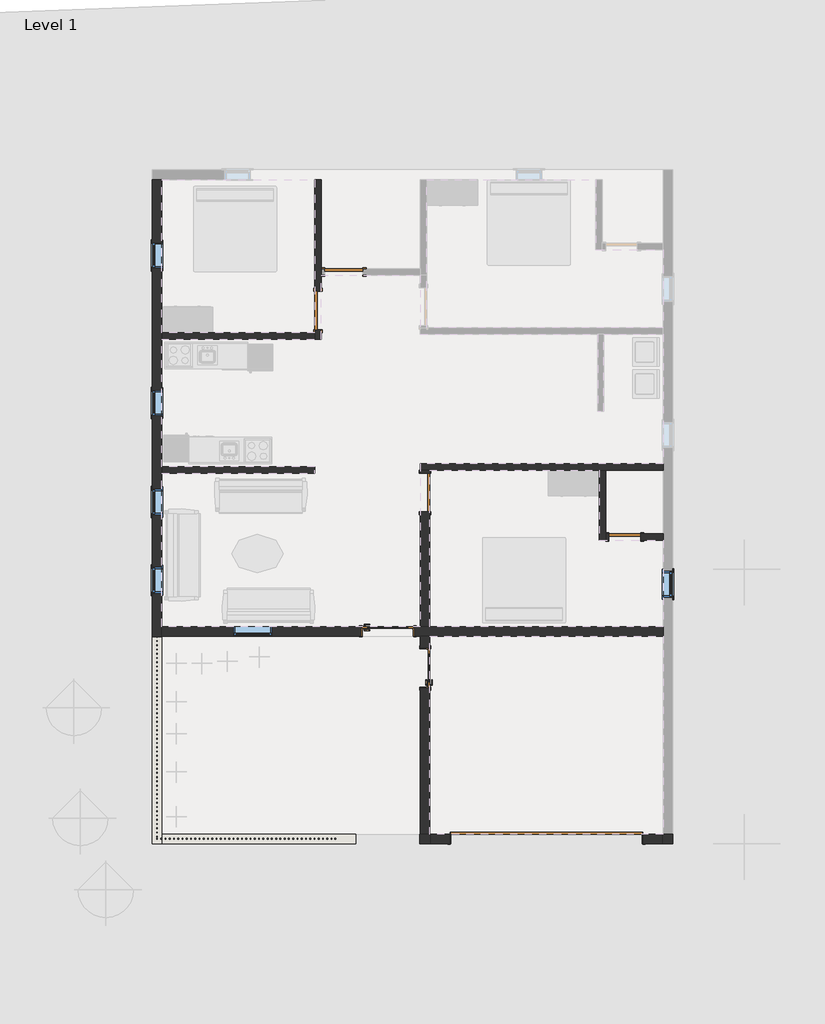
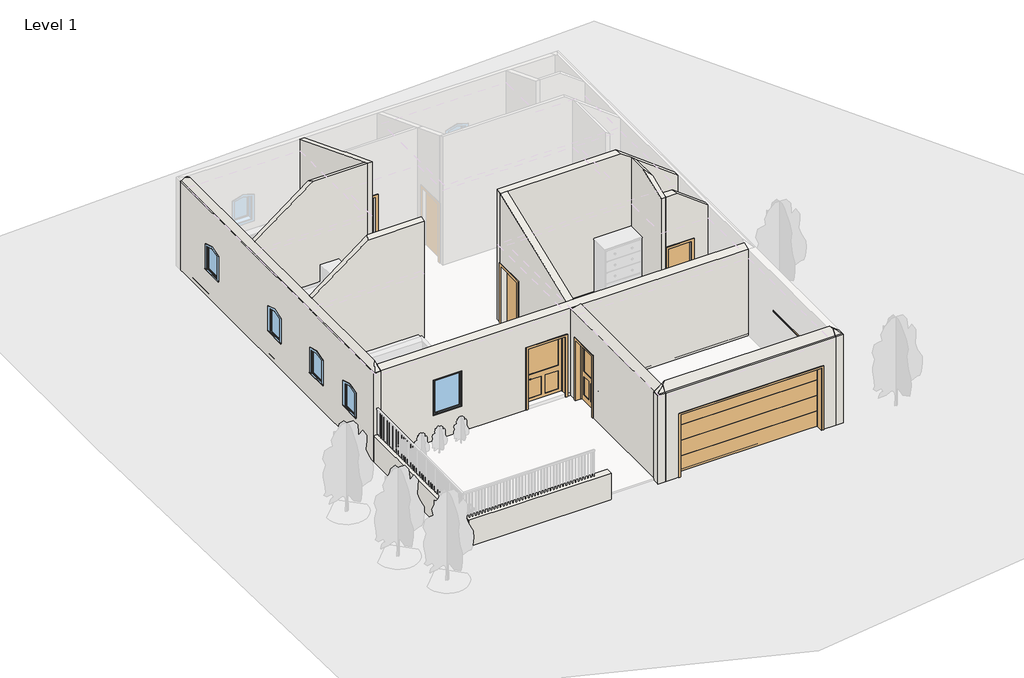
# One storey, part 1 of 3: 15 walls, 7 doors, 6 windows.
"""IFC4 building model written with IfcOpenShell, lengths in millimetres."""

from ifc_helpers import new_model, si_unit, frame, origin, origin_with_axes, place, context, project, spatial, polyline, circle_curve, outline, extrude, faceted_brep, transform, mapped, element, save
from ifc_brep_helpers import plane_surface, revolved_surface, advanced_brep
from components import door_b46a707d, door_4_f719ca0b, door_0f373a22, single_flush_25_e2b13fe9, door_a90ba1ad, door_686f89d2, window_fb83c811, window_c1f32544

model = new_model("IFC4")

# Units and contexts
model_context = context("Model", 3, world=origin())
ifc_project = project(units=[si_unit("LENGTHUNIT", "METRE", prefix="MILLI")], contexts=[model_context])

# Site, building, storey
site = spatial("IfcSite", under=ifc_project)
building = spatial("IfcBuilding", under=site)
storey = spatial("IfcBuildingStorey", under=building, Name="Level 1", Elevation=0.0)

# Doors
placement = place(None, origin())
door_shape = door_b46a707d(model_context)
element("IfcDoor", 1, ObjectType="36\" x 84\"", at=placement, inside=storey, context=model_context, shape_type="MappedRepresentation", body=[
    mapped(door_shape, transform((-6500.1618615, -2826.2329779, 0.0), x_axis=(0.0, -1.0, 0.0), y_axis=(1.0, 0.0, 0.0), z_axis=(0.0, 0.0, 1.0))),
])
door_4_shape = door_4_f719ca0b(model_context)
element("IfcDoor", 2, ObjectType="4'", at=placement, inside=storey, context=model_context, shape_type="MappedRepresentation", body=[
    mapped(door_4_shape, transform((-7392.3368615, -1946.7579779, 0.0), x_axis=(-1.0, 0.0, 0.0), y_axis=(0.0, -1.0, 0.0), z_axis=(0.0, 0.0, 1.0))),
])
door_2_shape = door_0f373a22(model_context)
element("IfcDoor", 3, ObjectType="Door-Garage-Flush_Panel : 180\" x 84\"", at=placement, inside=storey, context=model_context, shape_type="MappedRepresentation", body=[
    mapped(door_2_shape, transform((-3607.7368615, -6906.1079779, 0.0), x_axis=(-1.0, 0.0, 0.0), y_axis=(0.0, -1.0, 0.0), z_axis=(0.0, 0.0, 1.0))),
])
single_flush_25_shape = single_flush_25_e2b13fe9(model_context)
element("IfcDoor", 4, ObjectType="Single-Flush : 25'", at=placement, inside=storey, context=model_context, shape_type="MappedRepresentation", body=[
    mapped(single_flush_25_shape, transform((-1740.8368615, 297.9670221, 0.0), x_axis=(-1.0, 0.0, 0.0), y_axis=(0.0, -1.0, 0.0), z_axis=(0.0, 0.0, 1.0))),
])
door_3_shape = door_a90ba1ad(model_context)
element("IfcDoor", 5, ObjectType="Single-Flush : 36\" x 84\"", at=placement, inside=storey, context=model_context, shape_type="MappedRepresentation", body=[
    mapped(door_3_shape, transform((-6503.3368615, 1364.7670221, 0.0), x_axis=(0.0, 1.0, 0.0), y_axis=(-1.0, 0.0, 0.0), z_axis=(0.0, 0.0, 1.0))),
])
door_5_shape = door_686f89d2(model_context)
element("IfcDoor", 6, ObjectType="Single-Flush : 36\" x 84\"", at=placement, inside=storey, context=model_context, shape_type="MappedRepresentation", body=[
    mapped(door_5_shape, transform((-9056.0368615, 5708.1670221, 0.0), x_axis=(0.0, -1.0, 0.0), y_axis=(1.0, 0.0, 0.0), z_axis=(0.0, 0.0, 1.0))),
])
element("IfcDoor", 7, ObjectType="Single-Flush : 36\" x 84\"", at=placement, inside=storey, context=model_context, shape_type="MappedRepresentation", body=[
    mapped(door_5_shape, transform((-8446.4368615, 6622.5670221, 0.0), x_axis=(-1.0, 0.0, 0.0), y_axis=(0.0, -1.0, 0.0), z_axis=(0.0, 0.0, 1.0))),
])

# Walls
element("IfcWall", 8, ObjectType="6\"", at=placement, inside=storey, context=model_context, shape_type="Brep", body=[
    faceted_brep([(-9132.2368615, 5250.9670221, 2133.6), (-9132.2368615, 5250.9670221, 0.0), (-9132.2368615, 5174.7670221, 0.0), (-9132.2368615, 5022.3670221, 0.0), (-9132.2368615, 5022.3670221, 4617.2193535), (-9132.2368615, 5174.7670221, 4558.0035288), (-9132.2368615, 8832.3670221, 3136.823737), (-9132.2368615, 8832.3670221, 0.0), (-9132.2368615, 6165.3670221, 0.0), (-9132.2368615, 6165.3670221, 2133.6), (-8979.8368615, 5022.3670221, 0.0), (-8979.8368615, 5250.9670221, 0.0), (-8979.8368615, 5250.9670221, 2133.6), (-8979.8368615, 6165.3670221, 2133.6), (-8979.8368615, 6165.3670221, 0.0), (-8979.8368615, 6546.3670221, 0.0), (-8979.8368615, 6698.7670221, 0.0), (-8979.8368615, 8832.3670221, 0.0), (-8979.8368615, 8832.3670221, 3136.823737), (-8979.8368615, 6698.7670221, 3965.8452822), (-8979.8368615, 6546.3670221, 4025.0611069), (-8979.8368615, 5022.3670221, 4617.2193535)], [[[0, 1, 2, 3, 4, 5, 6, 7, 8, 9]], [[10, 11, 12, 13, 14, 15, 16, 17, 18, 19, 20, 21]], [[8, 7, 17, 16, 15, 14]], [[3, 2, 1, 11, 10]], [[7, 6, 18, 17]], [[4, 3, 10, 21]], [[12, 11, 1, 0]], [[13, 12, 0, 9]], [[14, 13, 9, 8]], [[6, 5, 4, 21, 20, 19, 18]]]),
])
element("IfcWall", 9, ObjectType="6\"", at=placement, inside=storey, context=model_context, shape_type="Brep", body=[
    faceted_brep([(-9132.2368615, 5174.7670221, 0.0), (-12789.8368615, 5174.7670221, 0.0), (-12789.8368615, 5174.7670221, 3192.4500731), (-10969.0989205, 5174.7670221, 4558.0035288), (-9132.2368615, 5174.7670221, 4558.0035288), (-9132.2368615, 5022.3670221, 0.0), (-9132.2368615, 5022.3670221, 4617.2193535), (-10890.1444876, 5022.3670221, 4617.2193535), (-12789.8368615, 5022.3670221, 3192.4500731), (-12789.8368615, 5022.3670221, 0.0)], [[[0, 1, 2, 3, 4]], [[5, 6, 7, 8, 9]], [[1, 0, 5, 9]], [[0, 4, 6, 5]], [[2, 1, 9, 8]], [[4, 3, 7, 6]], [[3, 2, 8, 7]]]),
])
element("IfcWall", 10, ObjectType="6\"", at=placement, inside=storey, context=model_context, shape_type="Brep", body=[
    faceted_brep([(-12789.8368615, 1821.9670221, 0.0), (-9132.2368615, 1821.9670221, 0.0), (-9132.2368615, 1821.9670221, 4558.0035288), (-10969.0989205, 1821.9670221, 4558.0035288), (-12789.8368615, 1821.9670221, 3192.4500731), (-12789.8368615, 1974.3670221, 0.0), (-12789.8368615, 1974.3670221, 3192.4500731), (-10890.1444876, 1974.3670221, 4617.2193535), (-9132.2368615, 1974.3670221, 4617.2193535), (-9132.2368615, 1974.3670221, 0.0)], [[[0, 1, 2, 3, 4]], [[5, 6, 7, 8, 9]], [[1, 0, 5, 9]], [[2, 1, 9, 8]], [[0, 4, 6, 5]], [[4, 3, 7, 6]], [[3, 2, 8, 7]]]),
])
element("IfcWall", 11, ObjectType="6\"", at=placement, inside=storey, context=model_context, shape_type="Brep", body=[
    faceted_brep([(-826.4368615, 2050.5670221, 0.0), (-6617.6368615, 2050.5670221, 0.0), (-6617.6368615, 2050.5670221, 4646.8272658), (-2765.6064518, 2050.5670221, 4646.8272658), (-826.4368615, 2050.5670221, 3192.4500731), (-826.4368615, 1898.1670221, 0.0), (-826.4368615, 1898.1670221, 3192.4500731), (-2198.0368615, 1898.1670221, 4221.1500731), (-2350.4368615, 1898.1670221, 4335.4500731), (-2686.652019, 1898.1670221, 4587.6114411), (-6389.0368615, 1898.1670221, 4587.6114411), (-6617.6368615, 1898.1670221, 4587.6114411), (-6617.6368615, 1898.1670221, 0.0), (-6389.0368615, 1898.1670221, 0.0), (-2350.4368615, 1898.1670221, 0.0), (-2198.0368615, 1898.1670221, 0.0)], [[[0, 1, 2, 3, 4]], [[5, 6, 7, 8, 9, 10, 11, 12, 13, 14, 15]], [[1, 0, 5, 15, 14, 13, 12]], [[0, 4, 6, 5]], [[2, 1, 12, 11]], [[4, 3, 9, 8, 7, 6]], [[3, 2, 11, 10, 9]]]),
])
element("IfcWall", 12, ObjectType="6\"", at=placement, inside=storey, context=model_context, shape_type="Brep", body=[
    faceted_brep([(-2350.4368615, 1898.1670221, 0.0), (-2350.4368615, 221.7670221, 0.0), (-2350.4368615, 221.7670221, 3936.2373699), (-2350.4368615, 1249.1953542, 4335.4500731), (-2350.4368615, 1898.1670221, 4335.4500731), (-2198.0368615, 1898.1670221, 0.0), (-2198.0368615, 1898.1670221, 4221.1500731), (-2198.0368615, 955.0287171, 4221.1500731), (-2198.0368615, 374.1670221, 3995.4531946), (-2198.0368615, 221.7670221, 3936.2373699), (-2198.0368615, 221.7670221, 0.0), (-2198.0368615, 374.1670221, 0.0)], [[[0, 1, 2, 3, 4]], [[5, 6, 7, 8, 9, 10, 11]], [[1, 0, 5, 11, 10]], [[2, 1, 10, 9]], [[0, 4, 6, 5]], [[4, 3, 7, 6]], [[3, 2, 9, 8, 7]]]),
])
element("IfcWall", 13, ObjectType="6\"", at=placement, inside=storey, context=model_context, shape_type="Brep", body=[
    faceted_brep([(-2198.0368615, 221.7670221, 0.0), (-2121.8368615, 221.7670221, 0.0), (-2121.8368615, 221.7670221, 2133.6), (-1359.8368615, 221.7670221, 2133.6), (-1359.8368615, 221.7670221, 0.0), (-826.4368615, 221.7670221, 0.0), (-826.4368615, 221.7670221, 3192.4500731), (-1818.1532573, 221.7670221, 3936.2373699), (-2198.0368615, 221.7670221, 3936.2373699), (-2121.8368615, 374.1670221, 2133.6), (-2121.8368615, 374.1670221, 0.0), (-2198.0368615, 374.1670221, 0.0), (-2198.0368615, 374.1670221, 3995.4531946), (-1897.1076902, 374.1670221, 3995.4531946), (-826.4368615, 374.1670221, 3192.4500731), (-826.4368615, 374.1670221, 0.0), (-1359.8368615, 374.1670221, 0.0), (-1359.8368615, 374.1670221, 2133.6)], [[[0, 1, 2, 3, 4, 5, 6, 7, 8]], [[9, 10, 11, 12, 13, 14, 15, 16, 17]], [[16, 15, 5, 4]], [[11, 10, 1, 0]], [[0, 8, 12, 11]], [[6, 5, 15, 14]], [[2, 1, 10, 9]], [[3, 2, 9, 17]], [[4, 3, 17, 16]], [[8, 7, 13, 12]], [[7, 6, 14, 13]]]),
])
element("IfcWall", 14, ObjectType="9\"", at=placement, inside=storey, context=model_context, shape_type="Brep", body=[
    faceted_brep([(-12789.8368615, -7017.2329779, 0.0), (-12789.8368615, -6788.6329779, 0.0), (-12789.8368615, -2076.9329779, 0.0), (-12789.8368615, -2076.9329779, 914.4), (-12789.8368615, -6788.6329779, 914.4), (-12789.8368615, -7017.2329779, 914.4), (-13018.4368615, -7017.2329779, 0.0), (-13018.4368615, -7017.2329779, 914.4), (-13018.4368615, -2076.9329779, 914.4), (-13018.4368615, -2076.9329779, 0.0)], [[[0, 1, 2, 3, 4, 5]], [[6, 7, 8, 9]], [[2, 1, 0, 6, 9]], [[3, 2, 9, 8]], [[5, 4, 3, 8, 7]], [[0, 5, 7, 6]]]),
])
element("IfcWall", 15, ObjectType="9\"", at=placement, inside=storey, context=model_context, shape_type="Brep", body=[
    faceted_brep([(-597.8368615, -6788.6329779, 0.0), (-826.4368615, -6788.6329779, 0.0), (-839.1368615, -6788.6329779, 0.0), (-839.1368615, -6788.6329779, 3228.975), (-597.8368615, -6788.6329779, 3048.0), (-597.8368615, -7017.2329779, 0.0), (-597.8368615, -7017.2329779, 3048.0), (-839.1368615, -7017.2329779, 3048.0), (-839.1368615, -7017.2329779, 0.0), (-839.1368615, -6967.118246, 3048.0), (-839.1368615, -6835.890869, 3228.975), (-597.8368615, -6967.118246, 3048.0)], [[[0, 1, 2, 3, 4]], [[5, 6, 7, 8]], [[2, 1, 0, 5, 8]], [[3, 2, 8, 7, 9, 10]], [[0, 4, 11, 6, 5]], [[4, 3, 10, 11]], [[10, 9, 11]], [[9, 7, 6, 11]]]),
])
element("IfcWall", 16, ObjectType="9\"", at=placement, inside=storey, context=model_context, shape_type="Brep", body=[
    faceted_brep([(-12789.8368615, -2064.2329779, 3048.0), (-12789.8368615, -2064.2329779, 0.0), (-8027.3368615, -2064.2329779, 0.0), (-8027.3368615, -2064.2329779, 2159.0), (-6757.3368615, -2064.2329779, 2159.0), (-6757.3368615, -2064.2329779, 0.0), (-6617.6368615, -2064.2329779, 0.0), (-6389.0368615, -2064.2329779, 0.0), (-826.4368615, -2064.2329779, 0.0), (-826.4368615, -2064.2329779, 3048.0), (-11075.3368615, -2064.2329779, 2133.6), (-10160.9368615, -2064.2329779, 2133.6), (-10160.9368615, -2064.2329779, 914.4), (-11075.3368615, -2064.2329779, 914.4), (-12789.8368615, -1835.6329779, 0.0), (-12789.8368615, -1835.6329779, 3136.823737), (-6617.6368615, -1835.6329779, 3136.823737), (-6389.0368615, -1835.6329779, 3136.823737), (-826.4368615, -1835.6329779, 3136.823737), (-826.4368615, -1835.6329779, 0.0), (-6389.0368615, -1835.6329779, 0.0), (-6617.6368615, -1835.6329779, 0.0), (-6757.3368615, -1835.6329779, 0.0), (-6757.3368615, -1835.6329779, 2159.0), (-8027.3368615, -1835.6329779, 2159.0), (-8027.3368615, -1835.6329779, 0.0), (-11075.3368615, -1835.6329779, 2133.6), (-11075.3368615, -1835.6329779, 914.4), (-10160.9368615, -1835.6329779, 914.4), (-10160.9368615, -1835.6329779, 2133.6)], [[[0, 1, 2, 3, 4, 5, 6, 7, 8, 9], [10, 11, 12, 13]], [[14, 15, 16, 17, 18, 19, 20, 21, 22, 23, 24, 25], [26, 27, 28, 29]], [[1, 14, 25, 2]], [[19, 8, 7, 6, 5, 22, 21, 20]], [[1, 0, 15, 14]], [[9, 8, 19, 18]], [[24, 3, 2, 25]], [[3, 24, 23, 4]], [[4, 23, 22, 5]], [[0, 9, 18, 17, 16, 15]], [[27, 26, 10, 13]], [[28, 27, 13, 12]], [[29, 28, 12, 11]], [[26, 29, 11, 10]]]),
])
element("IfcWall", 17, ObjectType="9\"", at=placement, inside=storey, context=model_context, shape_type="SweptSolid", body=[
    extrude(outline(polyline([(1898.1670221, 0.0), (1821.9670221, 0.0), (1821.9670221, 2133.6), (907.5670221, 2133.6), (907.5670221, 0.0), (-1835.6329779, 0.0), (-1835.6329779, 3136.823737), (1898.1670221, 4587.6114411), (1898.1670221, 0.0)])), frame((-6617.6368615, 0.0, 0.0), z_axis=(1.0, 0.0, 0.0), x_axis=(0.0, 1.0, 0.0)), (0.0, 0.0, 1.0), 228.6),
])
element("IfcWall", 18, ObjectType="9\"", at=placement, inside=storey, context=model_context, shape_type="Brep", body=[
    faceted_brep([(-6617.6368615, -2064.2329779, 3048.0), (-6617.6368615, -2064.2329779, 0.0), (-6617.6368615, -2343.6329779, 0.0), (-6617.6368615, -2343.6329779, 2159.0), (-6617.6368615, -3308.8329779, 2159.0), (-6617.6368615, -3308.8329779, 0.0), (-6617.6368615, -6788.6329779, 0.0), (-6617.6368615, -6788.6329779, 3048.0), (-6617.6368615, -2114.3477098, 3048.0), (-6389.0368615, -2064.2329779, 0.0), (-6389.0368615, -2064.2329779, 3048.0), (-6389.0368615, -2114.3477098, 3048.0), (-6389.0368615, -2238.6683827, 3219.45), (-6389.0368615, -6788.6329779, 3219.45), (-6389.0368615, -6788.6329779, 0.0), (-6389.0368615, -3308.8329779, 0.0), (-6389.0368615, -3308.8329779, 2159.0), (-6389.0368615, -2343.6329779, 2159.0), (-6389.0368615, -2343.6329779, 0.0)], [[[0, 1, 2, 3, 4, 5, 6, 7, 8]], [[9, 10, 11, 12, 13, 14, 15, 16, 17, 18]], [[1, 9, 18, 2]], [[14, 6, 5, 15]], [[1, 0, 10, 9]], [[7, 6, 14, 13]], [[4, 16, 15, 5]], [[16, 4, 3, 17]], [[17, 3, 2, 18]], [[10, 0, 8, 11]], [[7, 13, 12, 8]], [[12, 11, 8]]]),
])
element("IfcWall", 19, ObjectType="9\"", at=placement, inside=storey, context=model_context, shape_type="AdvancedBrep", body=[
    advanced_brep(
    [(-12789.8368615, -2076.9329779, 0.0), (-12789.8368615, -2064.2329779, 0.0), (-12789.8368615, -1835.6329779, 0.0), (-12789.8368615, 1821.9670221, 0.0), (-12789.8368615, 1974.3670221, 0.0), (-12789.8368615, 5022.3670221, 0.0), (-12789.8368615, 5174.7670221, 0.0), (-12789.8368615, 8832.3670221, 0.0), (-12789.8368615, 8832.3670221, 3136.823737), (-12789.8368615, 8689.2050605, 3192.4500731), (-12789.8368615, 5174.7670221, 3192.4500731), (-12789.8368615, 5022.3670221, 3192.4500731), (-12789.8368615, 1974.3670221, 3192.4500731), (-12789.8368615, 1821.9670221, 3192.4500731), (-12789.8368615, -1692.4710163, 3192.4500731), (-12789.8368615, -1835.6329779, 3136.823737), (-12789.8368615, -2064.2329779, 3048.0), (-12789.8368615, -2076.9329779, 3048.0), (-12789.8368615, -2076.9329779, 914.4), (-12789.8368615, -425.9329779, 1747.1290861), (-12789.8368615, -425.9329779, 914.4), (-12789.8368615, -1035.5329779, 914.4), (-12789.8368615, -1035.5329779, 1747.1290861), (-12789.8368615, -730.7329779, 1828.8), (-12789.8368615, 1440.9670221, 1747.1290861), (-12789.8368615, 1440.9670221, 914.4), (-12789.8368615, 831.3670221, 914.4), (-12789.8368615, 831.3670221, 1747.1290861), (-12789.8368615, 1136.1670221, 1828.8), (-12789.8368615, 3803.1670221, 1747.1290861), (-12789.8368615, 3803.1670221, 914.4), (-12789.8368615, 3193.5670221, 914.4), (-12789.8368615, 3193.5670221, 1747.1290861), (-12789.8368615, 3498.3670221, 1828.8), (-12789.8368615, 7327.4170221, 1747.1290861), (-12789.8368615, 7327.4170221, 914.4), (-12789.8368615, 6717.8170221, 914.4), (-12789.8368615, 6717.8170221, 1747.1290861), (-12789.8368615, 7022.6170221, 1828.8), (-13018.4368615, -2076.9329779, 0.0), (-13018.4368615, -2076.9329779, 914.4), (-13018.4368615, -2076.9329779, 3048.0), (-13018.4368615, -2064.2329779, 3048.0), (-13018.4368615, 8832.3670221, 3048.0), (-13018.4368615, 8832.3670221, 0.0), (-13018.4368615, -425.9329779, 1747.1290861), (-13018.4368615, -730.7329779, 1828.8), (-13018.4368615, -1035.5329779, 1747.1290861), (-13018.4368615, -1035.5329779, 914.4), (-13018.4368615, -425.9329779, 914.4), (-13018.4368615, 1440.9670221, 1747.1290861), (-13018.4368615, 1136.1670221, 1828.8), (-13018.4368615, 831.3670221, 1747.1290861), (-13018.4368615, 831.3670221, 914.4), (-13018.4368615, 1440.9670221, 914.4), (-13018.4368615, 3803.1670221, 1747.1290861), (-13018.4368615, 3498.3670221, 1828.8), (-13018.4368615, 3193.5670221, 1747.1290861), (-13018.4368615, 3193.5670221, 914.4), (-13018.4368615, 3803.1670221, 914.4), (-13018.4368615, 7327.4170221, 1747.1290861), (-13018.4368615, 7022.6170221, 1828.8), (-13018.4368615, 6717.8170221, 1747.1290861), (-13018.4368615, 6717.8170221, 914.4), (-13018.4368615, 7327.4170221, 914.4), (-12982.4369589, 8832.3670221, 3048.0), (-12864.0053096, 8832.3670221, 3136.823737), (-12982.4369589, -2064.2329779, 3048.0)],
    [
        (0, 1),
        (1, 2),
        (2, 3),
        (3, 4),
        (4, 5),
        (5, 6),
        (6, 7),
        (7, 8),
        (8, 9),
        (9, 10),
        (10, 11),
        (11, 12),
        (12, 13),
        (13, 14),
        (14, 15),
        (15, 16),
        (16, 17),
        (17, 18),
        (18, 0),
        (19, 20),
        (20, 21),
        (21, 22),
        (22, 23, circle_curve(frame((-12789.8368615, -730.7329779, 1219.2), z_axis=(-1.0, 0.0, 0.0), x_axis=(0.0, 1.0, 0.0)), 609.6)),
        (23, 19, circle_curve(frame((-12789.8368615, -730.7329779, 1219.2), z_axis=(-1.0, 0.0, 0.0), x_axis=(0.0, 1.0, 0.0)), 609.6)),
        (24, 25),
        (25, 26),
        (26, 27),
        (27, 28, circle_curve(frame((-12789.8368615, 1136.1670221, 1219.2), z_axis=(-1.0, 0.0, 0.0), x_axis=(0.0, 1.0, 0.0)), 609.6)),
        (28, 24, circle_curve(frame((-12789.8368615, 1136.1670221, 1219.2), z_axis=(-1.0, 0.0, 0.0), x_axis=(0.0, 1.0, 0.0)), 609.6)),
        (29, 30),
        (30, 31),
        (31, 32),
        (32, 33, circle_curve(frame((-12789.8368615, 3498.3670221, 1219.2), z_axis=(-1.0, 0.0, 0.0), x_axis=(0.0, 1.0, 0.0)), 609.6)),
        (33, 29, circle_curve(frame((-12789.8368615, 3498.3670221, 1219.2), z_axis=(-1.0, 0.0, 0.0), x_axis=(0.0, 1.0, 0.0)), 609.6)),
        (34, 35),
        (35, 36),
        (36, 37),
        (37, 38, circle_curve(frame((-12789.8368615, 7022.6170221, 1219.2), z_axis=(-1.0, 0.0, 0.0), x_axis=(0.0, 1.0, 0.0)), 609.6)),
        (38, 34, circle_curve(frame((-12789.8368615, 7022.6170221, 1219.2), z_axis=(-1.0, 0.0, 0.0), x_axis=(0.0, 1.0, 0.0)), 609.6)),
        (39, 40),
        (40, 41),
        (41, 42),
        (42, 43),
        (43, 44),
        (44, 39),
        (45, 46, circle_curve(frame((-13018.4368615, -730.7329779, 1219.2), z_axis=(1.0, 0.0, 0.0), x_axis=(0.0, 1.0, 0.0)), 609.6)),
        (46, 47, circle_curve(frame((-13018.4368615, -730.7329779, 1219.2), z_axis=(1.0, 0.0, 0.0), x_axis=(0.0, 1.0, 0.0)), 609.6)),
        (47, 48),
        (48, 49),
        (49, 45),
        (50, 51, circle_curve(frame((-13018.4368615, 1136.1670221, 1219.2), z_axis=(1.0, 0.0, 0.0), x_axis=(0.0, 1.0, 0.0)), 609.6)),
        (51, 52, circle_curve(frame((-13018.4368615, 1136.1670221, 1219.2), z_axis=(1.0, 0.0, 0.0), x_axis=(0.0, 1.0, 0.0)), 609.6)),
        (52, 53),
        (53, 54),
        (54, 50),
        (55, 56, circle_curve(frame((-13018.4368615, 3498.3670221, 1219.2), z_axis=(1.0, 0.0, 0.0), x_axis=(0.0, 1.0, 0.0)), 609.6)),
        (56, 57, circle_curve(frame((-13018.4368615, 3498.3670221, 1219.2), z_axis=(1.0, 0.0, 0.0), x_axis=(0.0, 1.0, 0.0)), 609.6)),
        (57, 58),
        (58, 59),
        (59, 55),
        (60, 61, circle_curve(frame((-13018.4368615, 7022.6170221, 1219.2), z_axis=(1.0, 0.0, 0.0), x_axis=(0.0, 1.0, 0.0)), 609.6)),
        (61, 62, circle_curve(frame((-13018.4368615, 7022.6170221, 1219.2), z_axis=(1.0, 0.0, 0.0), x_axis=(0.0, 1.0, 0.0)), 609.6)),
        (62, 63),
        (63, 64),
        (64, 60),
        (0, 39),
        (44, 7),
        (17, 41),
        (43, 65),
        (65, 66),
        (66, 8),
        (16, 67),
        (67, 42),
        (14, 67),
        (9, 66),
        (65, 67),
        (19, 45),
        (49, 20),
        (48, 21),
        (47, 22),
        (46, 23),
        (24, 50),
        (54, 25),
        (53, 26),
        (52, 27),
        (51, 28),
        (29, 55),
        (59, 30),
        (58, 31),
        (57, 32),
        (56, 33),
        (34, 60),
        (64, 35),
        (63, 36),
        (62, 37),
        (61, 38),
    ],
    [
        plane_surface(frame((-12789.8368615, 11385.0670221, 0.0), z_axis=(1.0, 0.0, 0.0), x_axis=(0.0, 1.0, 0.0))),
        plane_surface(frame((-13018.4368615, 11385.0670221, 0.0), z_axis=(-1.0, 0.0, 0.0), x_axis=(0.0, -1.0, 0.0))),
        plane_surface(frame((-12789.8368615, -2076.9329779, 0.0), z_axis=(0.0, 0.0, -1.0), x_axis=(-1.0, 0.0, 0.0))),
        plane_surface(frame((-12789.8368615, -2076.9329779, 3048.0), z_axis=(0.0, -1.0, 0.0), x_axis=(-1.0, 0.0, 0.0))),
        plane_surface(frame((-15342.5368615, 8832.3670221, 0.0), z_axis=(0.0, 1.0, 0.0), x_axis=(1.0, 0.0, 0.0))),
        plane_surface(frame((-12789.8368615, 8946.6670221, 3048.0), z_axis=(0.0, 0.0, 1.0), x_axis=(-1.0, 0.0, 0.0))),
        plane_surface(frame((-12982.4369589, -2064.2329779, 3048.0), z_axis=(0.0, -0.3621761357767551, 0.9321096752388195), x_axis=(1.0, 0.0, 0.0))),
        plane_surface(frame((-12982.4369589, 9060.9670221, 3048.0), z_axis=(-0.6000000000000011, 0.0, 0.7999999999999992), x_axis=(0.0, -1.0, 0.0))),
        plane_surface(frame((-633.8367641, 9060.9670221, 3048.0), z_axis=(0.0, 0.3621761357767564, 0.932109675238819), x_axis=(-1.0, 0.0, 0.0))),
        plane_surface(frame((-597.8368615, 9060.9670221, 3048.0), z_axis=(0.0, 0.0, 1.0), x_axis=(-1.0, 0.0, 0.0))),
        plane_surface(frame((-12789.8368615, -425.9329779, 1747.1290861), z_axis=(0.0, -1.0, 0.0), x_axis=(-1.0, 0.0, 0.0))),
        plane_surface(frame((-12789.8368615, -425.9329779, 914.4), z_axis=(0.0, 0.0, 1.0), x_axis=(-1.0, 0.0, 0.0))),
        plane_surface(frame((-12789.8368615, -1035.5329779, 914.4), z_axis=(0.0, 1.0, 0.0), x_axis=(-1.0, 0.0, 0.0))),
        revolved_surface(polyline([(-13018.4368615, -121.13297790000001, 1219.2), (-12789.8368615, -121.13297790000001, 1219.2)]), (-12789.8368615, -730.7329779, 1219.2), (-1.0, 0.0, 0.0)),
        plane_surface(frame((-12789.8368615, 1440.9670221, 1747.1290861), z_axis=(0.0, -1.0, 0.0), x_axis=(-1.0, 0.0, 0.0))),
        plane_surface(frame((-12789.8368615, 1440.9670221, 914.4), z_axis=(0.0, 0.0, 1.0), x_axis=(-1.0, 0.0, 0.0))),
        plane_surface(frame((-12789.8368615, 831.3670221, 914.4), z_axis=(0.0, 1.0, 0.0), x_axis=(-1.0, 0.0, 0.0))),
        revolved_surface(polyline([(-13018.4368615, 1745.7670220999998, 1219.2), (-12789.8368615, 1745.7670220999998, 1219.2)]), (-12789.8368615, 1136.1670221, 1219.2), (-1.0, 0.0, 0.0)),
        plane_surface(frame((-12789.8368615, 3803.1670221, 1747.1290861), z_axis=(0.0, -1.0, 0.0), x_axis=(-1.0, 0.0, 0.0))),
        plane_surface(frame((-12789.8368615, 3803.1670221, 914.4), z_axis=(0.0, 0.0, 1.0), x_axis=(-1.0, 0.0, 0.0))),
        plane_surface(frame((-12789.8368615, 3193.5670221, 914.4), z_axis=(0.0, 1.0, 0.0), x_axis=(-1.0, 0.0, 0.0))),
        revolved_surface(polyline([(-13018.4368615, 4107.967022100001, 1219.2), (-12789.8368615, 4107.967022100001, 1219.2)]), (-12789.8368615, 3498.3670221, 1219.2), (-1.0, 0.0, 0.0)),
        plane_surface(frame((-12789.8368615, 7327.4170221, 1747.1290861), z_axis=(0.0, -1.0, 0.0), x_axis=(-1.0, 0.0, 0.0))),
        plane_surface(frame((-12789.8368615, 7327.4170221, 914.4), z_axis=(0.0, 0.0, 1.0), x_axis=(-1.0, 0.0, 0.0))),
        plane_surface(frame((-12789.8368615, 6717.8170221, 914.4), z_axis=(0.0, 1.0, 0.0), x_axis=(-1.0, 0.0, 0.0))),
        revolved_surface(polyline([(-13018.4368615, 7632.217022100001, 1219.2), (-12789.8368615, 7632.217022100001, 1219.2)]), (-12789.8368615, 7022.6170221, 1219.2), (-1.0, 0.0, 0.0)),
    ],
    [
        (0, [[1, 2, 3, 4, 5, 6, 7, 8, 9, 10, 11, 12, 13, 14, 15, 16, 17, 18, 19], [20, 21, 22, 23, 24], [25, 26, 27, 28, 29], [30, 31, 32, 33, 34], [35, 36, 37, 38, 39]]),
        (1, [[40, 41, 42, 43, 44, 45], [46, 47, 48, 49, 50], [51, 52, 53, 54, 55], [56, 57, 58, 59, 60], [61, 62, 63, 64, 65]]),
        (2, [[-7, -6, -5, -4, -3, -2, -1, 66, -45, 67]]),
        (3, [[-19, -18, 68, -41, -40, -66]]),
        (4, [[-8, -67, -44, 69, 70, 71]]),
        (5, [[-17, 72, 73, -42, -68]]),
        (6, [[-16, -15, 74, -72]]),
        (7, [[-14, -13, -12, -11, -10, 75, -70, 76, -74]]),
        (8, [[-9, -71, -75]]),
        (9, [[-69, -43, -73, -76]]),
        (10, [[-20, 77, -50, 78]]),
        (11, [[-21, -78, -49, 79]]),
        (12, [[-22, -79, -48, 80]]),
        (13, [[-23, -80, -47, 81]]),
        (13, [[-24, -81, -46, -77]]),
        (14, [[-25, 82, -55, 83]]),
        (15, [[-26, -83, -54, 84]]),
        (16, [[-27, -84, -53, 85]]),
        (17, [[-28, -85, -52, 86]]),
        (17, [[-29, -86, -51, -82]]),
        (18, [[-30, 87, -60, 88]]),
        (19, [[-31, -88, -59, 89]]),
        (20, [[-32, -89, -58, 90]]),
        (21, [[-33, -90, -57, 91]]),
        (21, [[-34, -91, -56, -87]]),
        (22, [[-35, 92, -65, 93]]),
        (23, [[-36, -93, -64, 94]]),
        (24, [[-37, -94, -63, 95]]),
        (25, [[-38, -95, -62, 96]]),
        (25, [[-39, -96, -61, -92]]),
    ],
),
])
element("IfcWall", 20, ObjectType="9\"", at=placement, inside=storey, context=model_context, shape_type="Brep", body=[
    faceted_brep([(-6376.3368615, -6788.6329779, 0.0), (-6389.0368615, -6788.6329779, 0.0), (-6617.6368615, -6788.6329779, 0.0), (-6630.3368615, -6788.6329779, 0.0), (-6630.3368615, -6788.6329779, 3048.0), (-6617.6368615, -6788.6329779, 3048.0), (-6389.0368615, -6788.6329779, 3219.45), (-6376.3368615, -6788.6329779, 3228.975), (-6376.3368615, -7017.2329779, 0.0), (-6376.3368615, -7017.2329779, 3048.0), (-6617.6368615, -7017.2329779, 3048.0), (-6630.3368615, -7017.2329779, 3048.0), (-6630.3368615, -7017.2329779, 0.0), (-6376.3368615, -6835.890869, 3228.975), (-6376.3368615, -6967.118246, 3048.0), (-6617.6368615, -6967.118246, 3048.0)], [[[0, 1, 2, 3, 4, 5, 6, 7]], [[8, 9, 10, 11, 12]], [[3, 2, 1, 0, 8, 12]], [[4, 3, 12, 11]], [[0, 7, 13, 14, 9, 8]], [[5, 4, 11, 10, 15]], [[7, 6, 5, 15, 13]], [[15, 10, 9, 14]], [[14, 13, 15]]]),
])
element("IfcWall", 21, ObjectType="9\"", at=placement, inside=storey, context=model_context, shape_type="SweptSolid", body=[
    extrude(outline(polyline([(-12789.8368615, -6788.6329779), (-8154.3368615, -6788.6329779), (-8154.3368615, -7017.2329779), (-12789.8368615, -7017.2329779), (-12789.8368615, -6788.6329779)])), origin_with_axes(), (0.0, 0.0, 1.0), 914.4),
])
element("IfcWall", 22, ObjectType="9\"", at=placement, inside=storey, context=model_context, shape_type="Brep", body=[
    faceted_brep([(-839.1368615, -7017.2329779, 0.0), (-839.1368615, -7017.2329779, 3048.0), (-6376.3368615, -7017.2329779, 3048.0), (-6376.3368615, -7017.2329779, 0.0), (-5919.1368615, -7017.2329779, 0.0), (-5919.1368615, -7017.2329779, 2159.0), (-1296.3368615, -7017.2329779, 2159.0), (-1296.3368615, -7017.2329779, 0.0), (-839.1368615, -6788.6329779, 3228.975), (-839.1368615, -6788.6329779, 0.0), (-1296.3368615, -6788.6329779, 0.0), (-1296.3368615, -6788.6329779, 2159.0), (-5919.1368615, -6788.6329779, 2159.0), (-5919.1368615, -6788.6329779, 0.0), (-6376.3368615, -6788.6329779, 0.0), (-6376.3368615, -6788.6329779, 3228.975), (-6289.4393758, -6788.6329779, 3294.1481143), (-926.0343472, -6788.6329779, 3294.1481143), (-839.1368615, -6835.890869, 3228.975), (-839.1368615, -6967.118246, 3048.0), (-6376.3368615, -6967.118246, 3048.0), (-6376.3368615, -6835.890869, 3228.975)], [[[0, 1, 2, 3, 4, 5, 6, 7]], [[8, 9, 10, 11, 12, 13, 14, 15, 16, 17]], [[3, 14, 13, 4]], [[9, 0, 7, 10]], [[1, 0, 9, 8, 18, 19]], [[3, 2, 20, 21, 15, 14]], [[12, 5, 4, 13]], [[5, 12, 11, 6]], [[6, 11, 10, 7]], [[2, 1, 19, 20]], [[19, 18, 17, 16, 21, 20]], [[18, 8, 17]], [[16, 15, 21]]]),
])

# Windows
window_shape = window_fb83c811(model_context)
element("IfcWindow", 23, ObjectType="Archtop with Trim : 24\" x 36\"", at=placement, inside=storey, context=model_context, shape_type="MappedRepresentation", body=[
    mapped(window_shape, transform((-12904.1368615, -742.7132759, 0.0), x_axis=(0.0, 1.0, 0.0), y_axis=(-1.0, 0.0, 0.0), z_axis=(0.0, 0.0, 1.0))),
])
element("IfcWindow", 24, ObjectType="Archtop with Trim : 24\" x 36\"", at=placement, inside=storey, context=model_context, shape_type="MappedRepresentation", body=[
    mapped(window_shape, transform((-12904.1368615, 1124.1867241, 0.0), x_axis=(0.0, 1.0, 0.0), y_axis=(-1.0, 0.0, 0.0), z_axis=(0.0, 0.0, 1.0))),
])
element("IfcWindow", 25, ObjectType="Archtop with Trim : 24\" x 36\"", at=placement, inside=storey, context=model_context, shape_type="MappedRepresentation", body=[
    mapped(window_shape, transform((-12904.1368615, 3486.3867241, 0.0), x_axis=(0.0, 1.0, 0.0), y_axis=(-1.0, 0.0, 0.0), z_axis=(0.0, 0.0, 1.0))),
])
element("IfcWindow", 26, ObjectType="Archtop with Trim : 24\" x 36\"", at=placement, inside=storey, context=model_context, shape_type="MappedRepresentation", body=[
    mapped(window_shape, transform((-12904.1368615, 7010.6367241, 0.0), x_axis=(0.0, 1.0, 0.0), y_axis=(-1.0, 0.0, 0.0), z_axis=(0.0, 0.0, 1.0))),
])
element("IfcWindow", 27, ObjectType="Archtop with Trim : 24\" x 36\"", at=placement, inside=storey, context=model_context, shape_type="MappedRepresentation", body=[
    mapped(window_shape, transform((-712.1368615, -814.0026799, 0.0), x_axis=(0.0, -1.0, 0.0), y_axis=(1.0, 0.0, 0.0), z_axis=(0.0, 0.0, 1.0))),
])
window_2_shape = window_c1f32544(model_context)
element("IfcWindow", 28, ObjectType="Fixed : 36\" x 48\"", at=placement, inside=storey, context=model_context, shape_type="MappedRepresentation", body=[
    mapped(window_2_shape, transform((-10656.2368615, -1949.9329779, 0.0), x_axis=(-1.0, 0.0, 0.0), y_axis=(0.0, -1.0, 0.0), z_axis=(0.0, 0.0, 1.0))),
])

save(model, "model.ifc")

# Revit data of these elements
# Type "36\" x 84\""
#   Type Mark = "9"
#   Assembly Code = "B2030100"
#   Analytic Construction = "French door, wood frame with single glass"
#   Top Rail = 0' - 4 3/4"
#   Threshold Offset [instance default] = 0' - 0 1/2"
#   Thickness = 0' - 1 3/8"
#   Thermal Resistance (R) = 1.0696 (h·ft²·°F)/BTU
#   Swing Angle [instance default] = 90.00°
#   Stiles = 0' - 4 3/4"
#   Rough Width = 3' - 2"
#   Rough Height = 7' - 1"
#   Lock Rail = 0' - 7 1/8"
#   Height = 7' - 0"
#   Width = 3' - 0"
#   Heat Transfer Coefficient (U) = 0.9350 BTU/(h·ft²·°F)
#   Door Offset [instance default] = 0' - 0"
#   Bottom Rail = 0' - 9 1/2"
#   Threshold [instance default] = yes
#   Function = 1
#   Exterior Trim [instance default] = yes
#   Trim Material = Cherry
#   Threshold Material = Cherry
#   Panel Material = Cherry
#   Glazing = Glass
#   Frame Material = Cherry
#   Door Handle Material = Aluminum
#   Visual Light Transmittance = 0
#   Solar Heat Gain Coefficient = 0
#   Wall Closure = (empty or 0)
#   Construction Type = (empty or 0)
# Type "4'"
#   Type Mark = "10"
#   Assembly Code = "B2030100"
#   Analytic Construction = "French door, wood frame with single glass"
#   Top Rail = 0' - 4 3/4"
#   Threshold Offset [instance default] = 0' - 0 1/2"
#   Thickness = 0' - 1 3/8"
#   Thermal Resistance (R) = 1.0696 (h·ft²·°F)/BTU
#   Swing Angle [instance default] = 90.00°
#   Stiles = 0' - 4 3/4"
#   Rough Width = 4' - 2"
#   Rough Height = 7' - 1"
#   Lock Rail = 0' - 7 1/8"
#   Height = 7' - 0"
#   Width = 4' - 0"
#   Heat Transfer Coefficient (U) = 0.9350 BTU/(h·ft²·°F)
#   Door Offset [instance default] = 0' - 0"
#   Bottom Rail = 0' - 9 1/2"
#   Threshold [instance default] = yes
#   Function = 1
#   Exterior Trim [instance default] = yes
#   Trim Material = Cherry
#   Threshold Material = Cherry
#   Panel Material = Cherry
#   Glazing = Glass
#   Frame Material = Cherry
#   Door Handle Material = Aluminum
#   Visual Light Transmittance = 0
#   Solar Heat Gain Coefficient = 0
#   Wall Closure = (empty or 0)
#   Construction Type = (empty or 0)
# Type "Door-Garage-Flush_Panel : 180\" x 84\""
#   Type Mark = "12"
#   Assembly Code = "B2030400"
#   Analytic Construction = "Wooden"
#   Thickness = 0' - 1 1/2"
#   Thermal Resistance (R) = 2.5876 (h·ft²·°F)/BTU
#   Rough Width = 15' - 2"
#   Rough Height = 7' - 1"
#   Panel Height = 1' - 9"
#   Height = 7' - 0"
#   Width = 15' - 0"
#   Heat Transfer Coefficient (U) = 0.3865 BTU/(h·ft²·°F)
#   Function = 1
#   Exterior Trim [instance default] = yes
#   Trim Material = Cherry
#   Panel Material = Cherry
#   Frame Material = Cherry
#   Visual Light Transmittance = 0
#   Solar Heat Gain Coefficient = 0
#   Wall Closure = (empty or 0)
# Type "Single-Flush : 25'"
#   Type Mark = "8"
#   Construction Type Id = "MDOOR"
#   Assembly Code = "C1020"
#   Analytic Construction = "Metal"
#   Thickness = 0' - 2"
#   Heat Transfer Coefficient (U) = 0.651978 BTU/(h·ft²·°F)
#   Height = 7' - 0"
#   Trim Projection Ext = 0' - 1"
#   Trim Projection Int = 0' - 1"
#   Trim Width = 0' - 3"
#   Width = 2' - 6"
#   Define Thermal Properties by = 1
#   Door Material = Door - Panel
#   Frame Material = Door - Frame
#   Visual Light Transmittance = 0
#   Solar Heat Gain Coefficient = 0
#   Function = (empty or 0)
#   Wall Closure = (empty or 0)
# Type "Single-Flush : 36\" x 84\""
#   Type Mark = "1"
#   Construction Type Id = "MDOOR"
#   Assembly Code = "C1020"
#   Analytic Construction = "Metal"
#   Thickness = 0' - 2"
#   Heat Transfer Coefficient (U) = 0.651978 BTU/(h·ft²·°F)
#   Height = 7' - 0"
#   Trim Projection Ext = 0' - 1"
#   Trim Projection Int = 0' - 1"
#   Trim Width = 0' - 3"
#   Width = 3' - 0"
#   Define Thermal Properties by = 1
#   Door Material = Door - Panel
#   Frame Material = Door - Frame
#   Visual Light Transmittance = 0
#   Solar Heat Gain Coefficient = 0
#   Function = (empty or 0)
#   Wall Closure = (empty or 0)
# Type "6\""
#   Assembly Code = "B2010"
#   Layers, outside or top first: 0' - 6" "INT WALL" (function 1)
# Type "9\""
#   Assembly Code = "B2010"
#   Layers, outside or top first: 0' - 9" "EXT WALL" (function 1)
# Type "Archtop with Trim : 24\" x 36\""
#   Type Mark = "10"
#   Construction Type Id = "GSP4R"
#   Assembly Code = "B2020100"
#   Analytic Construction = "1/8 in Pilkington single glazing"
#   Visual Light Transmittance = 0.9
#   Solar Heat Gain Coefficient = 0.78
#   Heat Transfer Coefficient (U) = 0.6496 BTU/(h·ft²·°F)
#   Height = 3' - 0"
#   Radius = 2' - 0"
#   Default Sill Height = 3' - 0"
#   Trim Projection - Ext. = 0' - 0 1/2"
#   Trim Projection - Int. = 0' - 0 3/4"
#   Trim Width - Exterior = 0' - 3 1/2"
#   Trim Width - Interior = 0' - 3 1/2"
#   Width = 2' - 0"
#   Define Thermal Properties by = 1
#   Glass Pane Material = Glass
#   Sash Material = Sash
#   Trim Exterior Material = Trim
#   Trim Interior Material = Trim
#   Wall Closure = (empty or 0)
# Type "Fixed : 36\" x 48\""
#   Type Mark = "1"
#   Construction Type Id = "GSP4R"
#   Assembly Code = "B2020100"
#   Analytic Construction = "1/8 in Pilkington single glazing"
#   Visual Light Transmittance = 0.9
#   Solar Heat Gain Coefficient = 0.78
#   Heat Transfer Coefficient (U) = 0.6496 BTU/(h·ft²·°F)
#   Height = 4' - 0"
#   Default Sill Height = 3' - 0"
#   Width = 3' - 0"
#   Window Inset = 0' - 0 3/4"
#   Define Thermal Properties by = 1
#   Glass Pane Material = Glass
#   Sash Material = Sash
#   Wall Closure = (empty or 0)
# Element 1 (IfcDoor, "36\" x 84\"")
#   Threshold Offset = 0' - 0 1/2"
#   Swing Angle = 90.00°
#   Door Offset = 0' - 0"
#   Threshold = yes
#   Exterior Trim = yes
#   Phase Created = New Construction
#   Materials on its faces: "Cherry", "Aluminum", "Glass"
# Element 2 (IfcDoor, "4'")
#   Threshold Offset = 0' - 0 1/2"
#   Swing Angle = 90.00°
#   Door Offset = 0' - 0"
#   Threshold = yes
#   Exterior Trim = yes
#   Phase Created = New Construction
#   Materials on its faces: "Cherry", "Aluminum", "Glass"
# Element 3 (IfcDoor, "Door-Garage-Flush_Panel : 180\" x 84\"")
#   Exterior Trim = yes
#   Phase Created = New Construction
#   Materials on its faces: "Cherry"
# Element 4 (IfcDoor, "Single-Flush : 25'")
#   Phase Created = New Construction
#   Materials on its faces: "Door - Frame", "Door - Panel"
# Elements 5, 6, 7 (IfcDoor, "Single-Flush : 36\" x 84\"")
#   Phase Created = New Construction
#   Materials on its faces: "Door - Frame", "Door - Panel"
# Elements 8, 9, 10, 12, 13 (IfcWall, "6\"")
#   Top Offset = 0' - 0"
#   Base Offset = 0' - 0"
#   Unconnected Height = 10' - 0"
#   wall height = 10' - 0"
#   Phase Created = New Construction
#   Base Constraint = Level 1
#   Materials on its faces: "INT WALL"
# Element 11 (IfcWall, "6\"")
#   Top Offset = 0' - 0"
#   Base Offset = 0' - 0"
#   Unconnected Height = 10' - 0"
#   wall height = 10' - 0"
#   Phase Created = New Construction
#   Base Constraint = Level 1
#   Materials on its faces: "INT WALL", "EXT WALL"
# Elements 14, 21 (IfcWall, "9\"")
#   Top Offset = 0' - 0"
#   Base Offset = 0' - 0"
#   Unconnected Height = 3' - 0"
#   wall height = 3' - 0"
#   Phase Created = New Construction
#   Base Constraint = Level 1
#   Materials on its faces: "EXT WALL"
# Elements 15, 16, 17, 18, 19, 20, 22 (IfcWall, "9\"")
#   Top Offset = 0' - 0"
#   Base Offset = 0' - 0"
#   Unconnected Height = 10' - 0"
#   wall height = 10' - 0"
#   Phase Created = New Construction
#   Base Constraint = Level 1
#   Materials on its faces: "EXT WALL"
# Element 23 (IfcWindow, "Archtop with Trim : 24\" x 36\"")
#   Mark = "2"
#   Phase Created = New Construction
#   Materials on its faces: "Sash", "Trim", "Glass"
# Element 24 (IfcWindow, "Archtop with Trim : 24\" x 36\"")
#   Mark = "3"
#   Phase Created = New Construction
#   Materials on its faces: "Sash", "Trim", "Glass"
# Element 25 (IfcWindow, "Archtop with Trim : 24\" x 36\"")
#   Mark = "4"
#   Phase Created = New Construction
#   Materials on its faces: "Sash", "Trim", "Glass"
# Element 26 (IfcWindow, "Archtop with Trim : 24\" x 36\"")
#   Mark = "5"
#   Phase Created = New Construction
#   Materials on its faces: "Sash", "Trim", "Glass"
# Element 27 (IfcWindow, "Archtop with Trim : 24\" x 36\"")
#   Mark = "10"
#   Phase Created = New Construction
#   Materials on its faces: "Sash", "Trim", "Glass"
# Element 28 (IfcWindow, "Fixed : 36\" x 48\"")
#   Mark = "1"
#   Phase Created = New Construction
#   Materials on its faces: "Sash", "Glass"
# Materials
#   "Cherry": class "Wood", colour RGB 226 177 128, transparency 0, Description = "Prunus Serotina", Cost = 0
#   "Glass": class "Glass", colour RGB 0 128 192, transparency 0.75, Description = "Soda Lime Glass", Cost = 0
#   "Aluminum": class "Metal", colour RGB 247 247 247, transparency 0, Description = "Aluminum 6061", Cost = 0
#   "Door - Panel": class "Wood", colour RGB 210 159 95, transparency 0
#   "Door - Frame": colour RGB 118 70 51, transparency 0
#   "INT WALL": class "Generic", colour RGB 175 172 159, transparency 0, Cost = 0
#   "EXT WALL": class "Generic", colour RGB 216 216 204, transparency 0, Cost = 0
#   "Sash": class "Wood", colour RGB 224 178 126, transparency 0
#   "Trim": class "Wood", colour RGB 224 178 126, transparency 0
